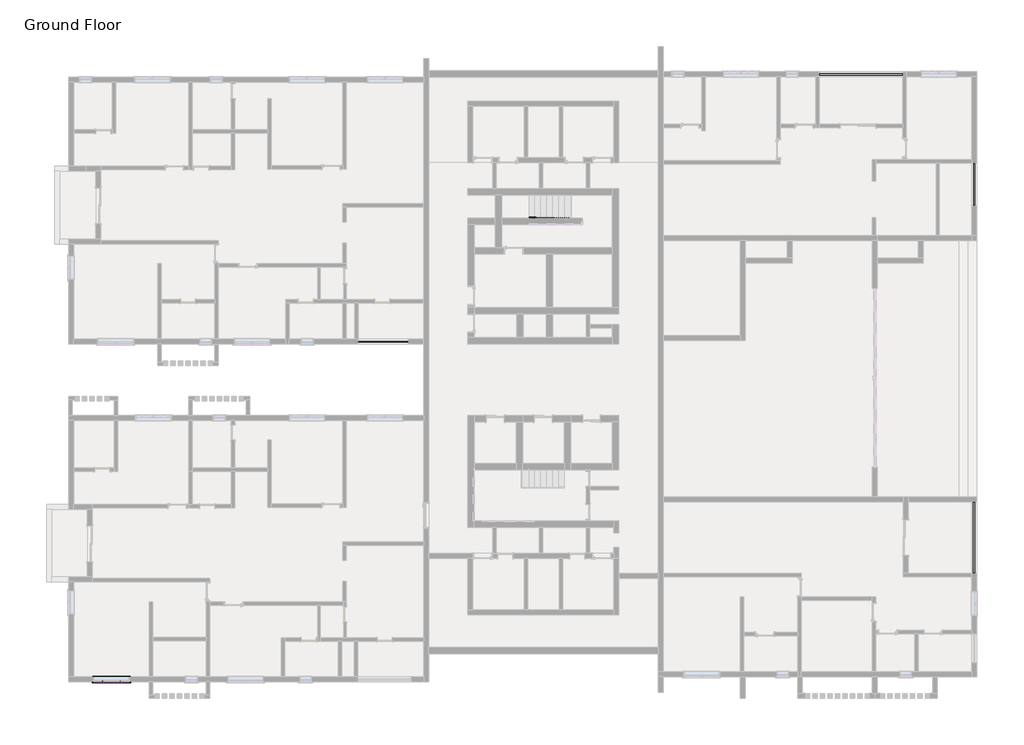
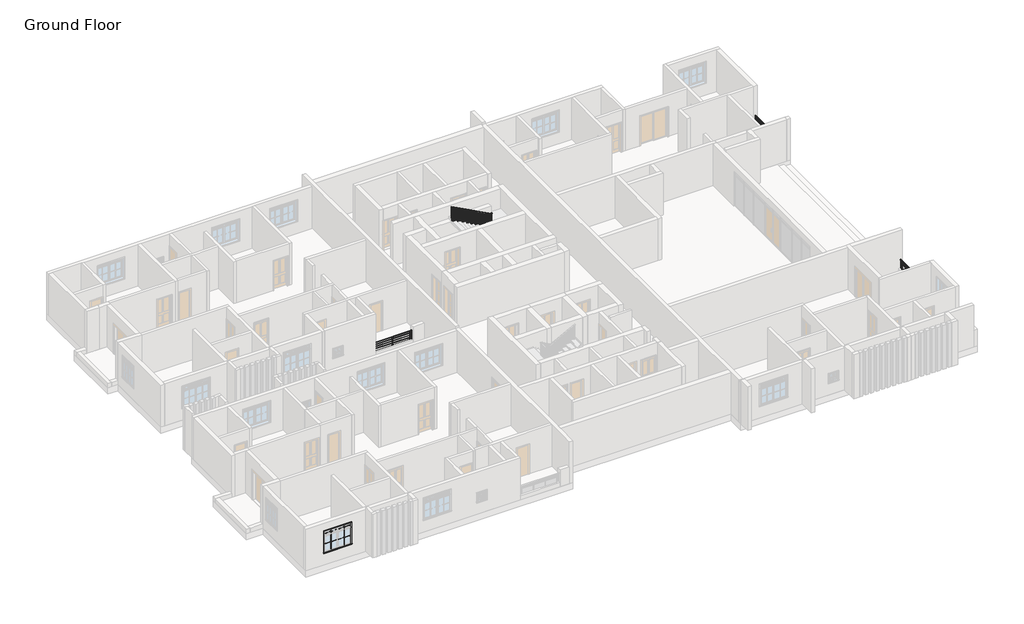
# One storey, part 7 of 9: 6 proxies, 5 railings.
"""IFC4 building model written with IfcOpenShell, lengths in millimetres."""

from ifc_helpers import new_model, si_unit, point, frame, frame_2d, origin, origin_with_axes, place, context, project, spatial, polyline, circle_curve, ellipse_curve, trimmed, segment, composite_curve, outline, extrude, faceted_brep, transform, mapped, element, save
from ifc_brep_helpers import plane_surface, extruded_surface, advanced_brep
from components import muntin_pattern_2x2_muntin_pattern_2x2_dc2504c2, muntin_pattern_2x2_muntin_pattern_2x2_0aa094e9, muntin_pattern_2x2_muntin_pattern_2x2_f17ebf58, trim_window_exterior_flat_with_sill_c22f0c79, trim_window_interior_flat_picture_frame_d1f4d6ef

model = new_model("IFC4")

# Units and contexts
model_context = context("Model", 3, world=origin())
ifc_project = project(units=[si_unit("LENGTHUNIT", "METRE", prefix="MILLI")], contexts=[model_context])

# Site, building, storey
site = spatial("IfcSite", under=ifc_project)
building = spatial("IfcBuilding", under=site)
storey = spatial("IfcBuildingStorey", under=building, Name="Ground Floor", Elevation=0.0)

# Proxies
placement = place(None, origin())
muntin_pattern_2x2_muntin_pattern_2x2_shape = muntin_pattern_2x2_muntin_pattern_2x2_dc2504c2(model_context)
element("IfcBuildingElementProxy", 1, Name="Muntin Pattern_2x2 : Muntin Pattern_2x2", ObjectType="Muntin Pattern_2x2 : Muntin Pattern_2x2", at=placement, inside=storey, context=model_context, shape_type="MappedRepresentation", body=[
    mapped(muntin_pattern_2x2_muntin_pattern_2x2_shape, transform((-11745.8828682, -1988.440108, 984.25), x_axis=(-1.0, 0.0, 0.0), y_axis=(0.0, -1.0, 0.0), z_axis=(0.0, 0.0, 1.0))),
])
muntin_pattern_2x2_muntin_pattern_2x2_2_shape = muntin_pattern_2x2_muntin_pattern_2x2_0aa094e9(model_context)
element("IfcBuildingElementProxy", 2, Name="Muntin Pattern_2x2 : Muntin Pattern_2x2", ObjectType="Muntin Pattern_2x2 : Muntin Pattern_2x2", at=placement, inside=storey, context=model_context, shape_type="MappedRepresentation", body=[
    mapped(muntin_pattern_2x2_muntin_pattern_2x2_2_shape, transform((-12657.1078682, -1988.440108, 984.25), x_axis=(1.0, 0.0, 0.0), y_axis=(0.0, 1.0, 0.0), z_axis=(0.0, 0.0, 1.0))),
])
muntin_pattern_2x2_muntin_pattern_2x2_3_shape = muntin_pattern_2x2_muntin_pattern_2x2_f17ebf58(model_context)
element("IfcBuildingElementProxy", 3, Name="Muntin Pattern_2x2 : Muntin Pattern_2x2", ObjectType="Muntin Pattern_2x2 : Muntin Pattern_2x2", at=placement, inside=storey, context=model_context, shape_type="MappedRepresentation", body=[
    mapped(muntin_pattern_2x2_muntin_pattern_2x2_3_shape, transform((-12657.1078682, -1988.440108, 2203.45), x_axis=(1.0, 0.0, 0.0), y_axis=(0.0, 1.0, 0.0), z_axis=(0.0, 0.0, 1.0))),
])
element("IfcBuildingElementProxy", 4, Name="Muntin Pattern_2x2 : Muntin Pattern_2x2", ObjectType="Muntin Pattern_2x2 : Muntin Pattern_2x2", at=placement, inside=storey, context=model_context, shape_type="MappedRepresentation", body=[
    mapped(muntin_pattern_2x2_muntin_pattern_2x2_3_shape, transform((-11745.8828682, -1988.440108, 2203.45), x_axis=(1.0, 0.0, 0.0), y_axis=(0.0, 1.0, 0.0), z_axis=(0.0, 0.0, 1.0))),
])
trim_window_exterior_flat_with_sill_shape = trim_window_exterior_flat_with_sill_c22f0c79(model_context)
element("IfcBuildingElementProxy", 5, Name="Trim-Window-Exterior-Flat : with Sill", ObjectType="Trim-Window-Exterior-Flat : with Sill", at=placement, inside=storey, context=model_context, shape_type="MappedRepresentation", body=[
    mapped(trim_window_exterior_flat_with_sill_shape, transform((-12201.4953682, -1997.965108, 2438.4), x_axis=(1.0, 0.0, 0.0), y_axis=(0.0, 0.0, 1.0), z_axis=(0.0, -1.0, 0.0))),
])
trim_window_interior_flat_picture_frame_shape = trim_window_interior_flat_picture_frame_d1f4d6ef(model_context)
element("IfcBuildingElementProxy", 6, Name="Trim-Window-Interior-Flat : Picture Frame", ObjectType="Trim-Window-Interior-Flat : Picture Frame", at=placement, inside=storey, context=model_context, shape_type="MappedRepresentation", body=[
    mapped(trim_window_interior_flat_picture_frame_shape, transform((-12201.4953682, -1743.965108, 2438.4), x_axis=(-1.0, 0.0, 0.0), y_axis=(0.0, 0.0, 1.0), z_axis=(0.0, 1.0, 0.0))),
])

# Railings
element("IfcRailing", 7, ObjectType="Glass Panel - Bottom Fill", at=placement, inside=storey, context=model_context, shape_type="SolidModel", body=[
    advanced_brep(
    [(31988.1546318, 7222.234892, 914.4), (31911.9546318, 7222.234892, 914.4), (31988.1546318, 3564.634892, 914.4), (31911.9546318, 3564.634892, 914.4)],
    [
        (0, 1, ellipse_curve(frame((31950.0546318, 7222.234892, 914.4), z_axis=(0.0, 1.0, 0.0), x_axis=(-1.0, 0.0, 0.0)), 38.1, 28.575)),
        (1, 0, ellipse_curve(frame((31950.0546318, 7222.234892, 914.4), z_axis=(0.0, 1.0, 0.0), x_axis=(-1.0, 0.0, 0.0)), 38.1, 28.575)),
        (2, 3, ellipse_curve(frame((31950.0546318, 3564.634892, 914.4), z_axis=(0.0, -1.0, 0.0), x_axis=(-1.0, 0.0, 0.0)), 38.1, 28.575)),
        (3, 2, ellipse_curve(frame((31950.0546318, 3564.634892, 914.4), z_axis=(0.0, -1.0, 0.0), x_axis=(-1.0, 0.0, 0.0)), 38.1, 28.575)),
        (0, 2),
        (3, 1),
    ],
    [
        plane_surface(frame((31950.0546318, 7222.234892, 914.4), z_axis=(0.0, 1.0, 0.0), x_axis=(0.0, 0.0, -1.0))),
        plane_surface(frame((31950.0546318, 3564.634892, 914.4), z_axis=(0.0, -1.0, 0.0), x_axis=(0.0, 0.0, -1.0))),
        extruded_surface(trimmed(ellipse_curve(frame((31950.0546318, 3564.634892, 914.4), z_axis=(0.0, 1.0, 0.0), x_axis=(-1.0, 0.0, 0.0)), 38.1, 28.575), [point((31988.1546318, 3564.634892, 914.4))], [point((31911.9546318, 3564.634892, 914.4))], True, "CARTESIAN"), (0.0, 3657.6000000000004, 0.0), 3657.6000000000004),
        extruded_surface(trimmed(ellipse_curve(frame((31950.0546318, 3564.634892, 914.4), z_axis=(0.0, 1.0, 0.0), x_axis=(-1.0, 0.0, 0.0)), 38.1, 28.575), [point((31911.9546318, 3564.634892, 914.4))], [point((31988.1546318, 3564.634892, 914.4))], True, "CARTESIAN"), (0.0, 3657.6000000000004, 0.0), 3657.6000000000004),
    ],
    [
        (0, [[1, 2]]),
        (1, [[3, 4]]),
        (2, [[-1, 5, -4, 6]]),
        (3, [[-2, -6, -3, -5]]),
    ],
),
    extrude(outline(polyline([(31937.3546318, 7222.234892), (31962.7546318, 7222.234892), (31962.7546318, 3564.634892), (31937.3546318, 3564.634892), (31937.3546318, 7222.234892)])), frame((0.0, 0.0, 800.1), z_axis=(0.0, 0.0, 1.0), x_axis=(1.0, 0.0, 0.0)), (0.0, 0.0, 1.0), 25.4),
    extrude(outline(polyline([(31937.3546318, 7222.234892), (31962.7546318, 7222.234892), (31962.7546318, 3564.634892), (31937.3546318, 3564.634892), (31937.3546318, 7222.234892)])), frame((0.0, 0.0, 698.5), z_axis=(0.0, 0.0, 1.0), x_axis=(1.0, 0.0, 0.0)), (0.0, 0.0, 1.0), 25.4),
    extrude(outline(polyline([(31924.6546318, 3774.184892), (31975.4546318, 3774.184892), (31975.4546318, 3761.484892), (31924.6546318, 3761.484892), (31924.6546318, 3774.184892)])), origin_with_axes(), (0.0, 0.0, 1.0), 885.825),
    extrude(outline(polyline([(31956.5897888, 4580.634892), (31956.5897888, 3767.834892), (31950.2397888, 3767.834892), (31950.2397888, 4580.634892), (31956.5897888, 4580.634892)])), frame((0.0, 0.0, 101.6), z_axis=(0.0, 0.0, 1.0), x_axis=(1.0, 0.0, 0.0)), (0.0, 0.0, 1.0), 596.9),
    extrude(outline(polyline([(31924.6546318, 4586.984892), (31975.4546318, 4586.984892), (31975.4546318, 4574.284892), (31924.6546318, 4574.284892), (31924.6546318, 4586.984892)])), origin_with_axes(), (0.0, 0.0, 1.0), 885.825),
    extrude(outline(polyline([(31956.5897888, 5393.434892), (31956.5897888, 4580.634892), (31950.2397888, 4580.634892), (31950.2397888, 5393.434892), (31956.5897888, 5393.434892)])), frame((0.0, 0.0, 101.6), z_axis=(0.0, 0.0, 1.0), x_axis=(1.0, 0.0, 0.0)), (0.0, 0.0, 1.0), 596.9),
    extrude(outline(polyline([(31924.6546318, 5399.784892), (31975.4546318, 5399.784892), (31975.4546318, 5387.084892), (31924.6546318, 5387.084892), (31924.6546318, 5399.784892)])), origin_with_axes(), (0.0, 0.0, 1.0), 885.825),
    extrude(outline(polyline([(31956.5897888, 6206.234892), (31956.5897888, 5393.434892), (31950.2397888, 5393.434892), (31950.2397888, 6206.234892), (31956.5897888, 6206.234892)])), frame((0.0, 0.0, 101.6), z_axis=(0.0, 0.0, 1.0), x_axis=(1.0, 0.0, 0.0)), (0.0, 0.0, 1.0), 596.9),
    extrude(outline(polyline([(31924.6546318, 6212.584892), (31975.4546318, 6212.584892), (31975.4546318, 6199.884892), (31924.6546318, 6199.884892), (31924.6546318, 6212.584892)])), origin_with_axes(), (0.0, 0.0, 1.0), 885.825),
    extrude(outline(polyline([(31956.5897888, 7019.034892), (31956.5897888, 6206.234892), (31950.2397888, 6206.234892), (31950.2397888, 7019.034892), (31956.5897888, 7019.034892)])), frame((0.0, 0.0, 101.6), z_axis=(0.0, 0.0, 1.0), x_axis=(1.0, 0.0, 0.0)), (0.0, 0.0, 1.0), 596.9),
    extrude(outline(polyline([(31924.6546318, 7025.384892), (31975.4546318, 7025.384892), (31975.4546318, 7012.684892), (31924.6546318, 7012.684892), (31924.6546318, 7025.384892)])), origin_with_axes(), (0.0, 0.0, 1.0), 885.825),
    extrude(outline(polyline([(31940.5296318, 3577.334892), (31959.5796318, 3577.334892), (31959.5796318, 3558.284892), (31940.5296318, 3558.284892), (31940.5296318, 3577.334892)])), origin_with_axes(), (0.0, 0.0, 1.0), 885.825),
    extrude(outline(polyline([(31940.5296318, 7228.584892), (31959.5796318, 7228.584892), (31959.5796318, 7209.534892), (31940.5296318, 7209.534892), (31940.5296318, 7228.584892)])), origin_with_axes(), (0.0, 0.0, 1.0), 885.825),
])
element("IfcRailing", 8, ObjectType="Glass Panel - Bottom Fill", at=placement, inside=storey, context=model_context, shape_type="SolidModel", body=[
    advanced_brep(
    [(23936.3546318, 29155.134892, 914.4), (23936.3546318, 29078.934892, 914.4), (28292.4546318, 29155.134892, 914.4), (28292.4546318, 29078.934892, 914.4)],
    [
        (0, 1, ellipse_curve(frame((23936.3546318, 29117.034892, 914.4), z_axis=(-1.0, 0.0, 0.0), x_axis=(0.0, -1.0, 0.0)), 38.1, 28.575)),
        (1, 0, ellipse_curve(frame((23936.3546318, 29117.034892, 914.4), z_axis=(-1.0, 0.0, 0.0), x_axis=(0.0, -1.0, 0.0)), 38.1, 28.575)),
        (2, 3, ellipse_curve(frame((28292.4546318, 29117.034892, 914.4), z_axis=(1.0, 0.0, 0.0), x_axis=(0.0, -1.0, 0.0)), 38.1, 28.575)),
        (3, 2, ellipse_curve(frame((28292.4546318, 29117.034892, 914.4), z_axis=(1.0, 0.0, 0.0), x_axis=(0.0, -1.0, 0.0)), 38.1, 28.575)),
        (0, 2),
        (3, 1),
    ],
    [
        plane_surface(frame((23936.3546318, 29117.034892, 914.4), z_axis=(-1.0, 0.0, 0.0), x_axis=(0.0, 1.0, 0.0))),
        plane_surface(frame((28292.4546318, 29117.034892, 914.4), z_axis=(1.0, 0.0, 0.0), x_axis=(0.0, 1.0, 0.0))),
        extruded_surface(trimmed(ellipse_curve(frame((28292.4546318, 29117.034892, 914.4), z_axis=(-1.0, 0.0, 0.0), x_axis=(0.0, -1.0, 0.0)), 38.1, 28.575), [point((28292.4546318, 29155.134892, 914.4))], [point((28292.4546318, 29078.934892, 914.4))], True, "CARTESIAN"), (-4356.0999999999985, 0.0, 0.0), 4356.0999999999985),
        extruded_surface(trimmed(ellipse_curve(frame((28292.4546318, 29117.034892, 914.4), z_axis=(-1.0, 0.0, 0.0), x_axis=(0.0, -1.0, 0.0)), 38.1, 28.575), [point((28292.4546318, 29078.934892, 914.4))], [point((28292.4546318, 29155.134892, 914.4))], True, "CARTESIAN"), (-4356.0999999999985, 0.0, 0.0), 4356.0999999999985),
    ],
    [
        (0, [[1, 2]]),
        (1, [[3, 4]]),
        (2, [[-1, 5, -4, 6]]),
        (3, [[-2, -6, -3, -5]]),
    ],
),
    extrude(outline(polyline([(23936.3546318, 29104.334892), (23936.3546318, 29129.734892), (28292.4546318, 29129.734892), (28292.4546318, 29104.334892), (23936.3546318, 29104.334892)])), frame((0.0, 0.0, 800.1), z_axis=(0.0, 0.0, 1.0), x_axis=(1.0, 0.0, 0.0)), (0.0, 0.0, 1.0), 25.4),
    extrude(outline(polyline([(23936.3546318, 29104.334892), (23936.3546318, 29129.734892), (28292.4546318, 29129.734892), (28292.4546318, 29104.334892), (23936.3546318, 29104.334892)])), frame((0.0, 0.0, 698.5), z_axis=(0.0, 0.0, 1.0), x_axis=(1.0, 0.0, 0.0)), (0.0, 0.0, 1.0), 25.4),
    extrude(outline(polyline([(28140.0546318, 29091.634892), (28140.0546318, 29142.434892), (28152.7546318, 29142.434892), (28152.7546318, 29091.634892), (28140.0546318, 29091.634892)])), origin_with_axes(), (0.0, 0.0, 1.0), 885.825),
    extrude(outline(polyline([(27333.6046318, 29123.570049), (28146.4046318, 29123.570049), (28146.4046318, 29117.220049), (27333.6046318, 29117.220049), (27333.6046318, 29123.570049)])), frame((0.0, 0.0, 101.6), z_axis=(0.0, 0.0, 1.0), x_axis=(1.0, 0.0, 0.0)), (0.0, 0.0, 1.0), 596.9),
    extrude(outline(polyline([(27327.2546318, 29091.634892), (27327.2546318, 29142.434892), (27339.9546318, 29142.434892), (27339.9546318, 29091.634892), (27327.2546318, 29091.634892)])), origin_with_axes(), (0.0, 0.0, 1.0), 885.825),
    extrude(outline(polyline([(26520.8046318, 29123.570049), (27333.6046318, 29123.570049), (27333.6046318, 29117.220049), (26520.8046318, 29117.220049), (26520.8046318, 29123.570049)])), frame((0.0, 0.0, 101.6), z_axis=(0.0, 0.0, 1.0), x_axis=(1.0, 0.0, 0.0)), (0.0, 0.0, 1.0), 596.9),
    extrude(outline(polyline([(26514.4546318, 29091.634892), (26514.4546318, 29142.434892), (26527.1546318, 29142.434892), (26527.1546318, 29091.634892), (26514.4546318, 29091.634892)])), origin_with_axes(), (0.0, 0.0, 1.0), 885.825),
    extrude(outline(polyline([(25708.0046318, 29123.570049), (26520.8046318, 29123.570049), (26520.8046318, 29117.220049), (25708.0046318, 29117.220049), (25708.0046318, 29123.570049)])), frame((0.0, 0.0, 101.6), z_axis=(0.0, 0.0, 1.0), x_axis=(1.0, 0.0, 0.0)), (0.0, 0.0, 1.0), 596.9),
    extrude(outline(polyline([(25701.6546318, 29091.634892), (25701.6546318, 29142.434892), (25714.3546318, 29142.434892), (25714.3546318, 29091.634892), (25701.6546318, 29091.634892)])), origin_with_axes(), (0.0, 0.0, 1.0), 885.825),
    extrude(outline(polyline([(24895.2046318, 29123.570049), (25708.0046318, 29123.570049), (25708.0046318, 29117.220049), (24895.2046318, 29117.220049), (24895.2046318, 29123.570049)])), frame((0.0, 0.0, 101.6), z_axis=(0.0, 0.0, 1.0), x_axis=(1.0, 0.0, 0.0)), (0.0, 0.0, 1.0), 596.9),
    extrude(outline(polyline([(24888.8546318, 29091.634892), (24888.8546318, 29142.434892), (24901.5546318, 29142.434892), (24901.5546318, 29091.634892), (24888.8546318, 29091.634892)])), origin_with_axes(), (0.0, 0.0, 1.0), 885.825),
    extrude(outline(polyline([(24082.4046318, 29123.570049), (24895.2046318, 29123.570049), (24895.2046318, 29117.220049), (24082.4046318, 29117.220049), (24082.4046318, 29123.570049)])), frame((0.0, 0.0, 101.6), z_axis=(0.0, 0.0, 1.0), x_axis=(1.0, 0.0, 0.0)), (0.0, 0.0, 1.0), 596.9),
    extrude(outline(polyline([(24076.0546318, 29091.634892), (24076.0546318, 29142.434892), (24088.7546318, 29142.434892), (24088.7546318, 29091.634892), (24076.0546318, 29091.634892)])), origin_with_axes(), (0.0, 0.0, 1.0), 885.825),
    extrude(outline(polyline([(28279.7546318, 29107.509892), (28279.7546318, 29126.559892), (28298.8046318, 29126.559892), (28298.8046318, 29107.509892), (28279.7546318, 29107.509892)])), origin_with_axes(), (0.0, 0.0, 1.0), 885.825),
    extrude(outline(polyline([(23930.0046318, 29107.509892), (23930.0046318, 29126.559892), (23949.0546318, 29126.559892), (23949.0546318, 29107.509892), (23930.0046318, 29107.509892)])), origin_with_axes(), (0.0, 0.0, 1.0), 885.825),
])
element("IfcRailing", 9, ObjectType="Handrail - Pipe", at=placement, inside=storey, context=model_context, shape_type="SweptSolid", body=[
    extrude(outline(composite_curve([segment(trimmed(circle_curve(frame_2d((15426.434892, 895.35)), 19.05), [point((15407.384892, 895.35))], [point((15445.484892, 895.35))], False, "CARTESIAN"), True, "CONTINUOUS"), segment(trimmed(circle_curve(frame_2d((15426.434892, 895.35)), 19.05), [point((15445.484892, 895.35))], [point((15407.384892, 895.35))], False, "CARTESIAN"), True, "CONTINUOUS")], self_intersect=False)), frame((428.6546318, 0.0, 0.0), z_axis=(1.0, 0.0, 0.0), x_axis=(0.0, 1.0, 0.0)), (0.0, 0.0, 1.0), 2565.4),
    extrude(outline(composite_curve([segment(trimmed(circle_curve(frame_2d((15426.434892, 749.3)), 12.7), [point((15439.134892, 749.3))], [point((15413.734892, 749.3))], False, "CARTESIAN"), True, "CONTINUOUS"), segment(trimmed(circle_curve(frame_2d((15426.434892, 749.3)), 12.7), [point((15413.734892, 749.3))], [point((15439.134892, 749.3))], False, "CARTESIAN"), True, "CONTINUOUS")], self_intersect=False)), frame((428.6546318, 0.0, 0.0), z_axis=(1.0, 0.0, 0.0), x_axis=(0.0, 1.0, 0.0)), (0.0, 0.0, 1.0), 2565.4),
    extrude(outline(composite_curve([segment(trimmed(circle_curve(frame_2d((15426.434892, 596.9)), 12.7), [point((15439.134892, 596.9))], [point((15413.734892, 596.9))], False, "CARTESIAN"), True, "CONTINUOUS"), segment(trimmed(circle_curve(frame_2d((15426.434892, 596.9)), 12.7), [point((15413.734892, 596.9))], [point((15439.134892, 596.9))], False, "CARTESIAN"), True, "CONTINUOUS")], self_intersect=False)), frame((428.6546318, 0.0, 0.0), z_axis=(1.0, 0.0, 0.0), x_axis=(0.0, 1.0, 0.0)), (0.0, 0.0, 1.0), 2565.4),
    extrude(outline(composite_curve([segment(trimmed(circle_curve(frame_2d((15426.434892, 444.5)), 12.7), [point((15439.134892, 444.5))], [point((15413.734892, 444.5))], False, "CARTESIAN"), True, "CONTINUOUS"), segment(trimmed(circle_curve(frame_2d((15426.434892, 444.5)), 12.7), [point((15413.734892, 444.5))], [point((15439.134892, 444.5))], False, "CARTESIAN"), True, "CONTINUOUS")], self_intersect=False)), frame((428.6546318, 0.0, 0.0), z_axis=(1.0, 0.0, 0.0), x_axis=(0.0, 1.0, 0.0)), (0.0, 0.0, 1.0), 2565.4),
    extrude(outline(composite_curve([segment(trimmed(circle_curve(frame_2d((15426.434892, 292.1)), 12.7), [point((15439.134892, 292.1))], [point((15413.734892, 292.1))], False, "CARTESIAN"), True, "CONTINUOUS"), segment(trimmed(circle_curve(frame_2d((15426.434892, 292.1)), 12.7), [point((15413.734892, 292.1))], [point((15439.134892, 292.1))], False, "CARTESIAN"), True, "CONTINUOUS")], self_intersect=False)), frame((428.6546318, 0.0, 0.0), z_axis=(1.0, 0.0, 0.0), x_axis=(0.0, 1.0, 0.0)), (0.0, 0.0, 1.0), 2565.4),
    extrude(outline(composite_curve([segment(trimmed(circle_curve(frame_2d((15426.434892, 139.7)), 12.7), [point((15439.134892, 139.7))], [point((15413.734892, 139.7))], False, "CARTESIAN"), True, "CONTINUOUS"), segment(trimmed(circle_curve(frame_2d((15426.434892, 139.7)), 12.7), [point((15413.734892, 139.7))], [point((15439.134892, 139.7))], False, "CARTESIAN"), True, "CONTINUOUS")], self_intersect=False)), frame((428.6546318, 0.0, 0.0), z_axis=(1.0, 0.0, 0.0), x_axis=(0.0, 1.0, 0.0)), (0.0, 0.0, 1.0), 2565.4),
    extrude(outline(composite_curve([segment(trimmed(circle_curve(frame_2d((2867.0546318, 15426.434892)), 12.7), [point((2867.0546318, 15439.134892))], [point((2867.0546318, 15413.734892))], False, "CARTESIAN"), True, "CONTINUOUS"), segment(trimmed(circle_curve(frame_2d((2867.0546318, 15426.434892)), 12.7), [point((2867.0546318, 15413.734892))], [point((2867.0546318, 15439.134892))], False, "CARTESIAN"), True, "CONTINUOUS")], self_intersect=False)), origin_with_axes(), (0.0, 0.0, 1.0), 876.3),
    extrude(outline(composite_curve([segment(trimmed(circle_curve(frame_2d((1647.8546318, 15426.434892)), 12.7), [point((1647.8546318, 15439.134892))], [point((1647.8546318, 15413.734892))], False, "CARTESIAN"), True, "CONTINUOUS"), segment(trimmed(circle_curve(frame_2d((1647.8546318, 15426.434892)), 12.7), [point((1647.8546318, 15413.734892))], [point((1647.8546318, 15439.134892))], False, "CARTESIAN"), True, "CONTINUOUS")], self_intersect=False)), origin_with_axes(), (0.0, 0.0, 1.0), 876.3),
    extrude(outline(composite_curve([segment(trimmed(circle_curve(frame_2d((2981.3546318, 15426.434892)), 12.7), [point((2981.3546318, 15439.134892))], [point((2981.3546318, 15413.734892))], False, "CARTESIAN"), True, "CONTINUOUS"), segment(trimmed(circle_curve(frame_2d((2981.3546318, 15426.434892)), 12.7), [point((2981.3546318, 15413.734892))], [point((2981.3546318, 15439.134892))], False, "CARTESIAN"), True, "CONTINUOUS")], self_intersect=False)), origin_with_axes(), (0.0, 0.0, 1.0), 876.3),
    extrude(outline(composite_curve([segment(trimmed(circle_curve(frame_2d((441.3546318, 15426.434892)), 12.7), [point((441.3546318, 15439.134892))], [point((441.3546318, 15413.734892))], False, "CARTESIAN"), True, "CONTINUOUS"), segment(trimmed(circle_curve(frame_2d((441.3546318, 15426.434892)), 12.7), [point((441.3546318, 15413.734892))], [point((441.3546318, 15439.134892))], False, "CARTESIAN"), True, "CONTINUOUS")], self_intersect=False)), origin_with_axes(), (0.0, 0.0, 1.0), 876.3),
])
element("IfcRailing", 10, ObjectType="Handrail - Pipe", at=placement, inside=storey, context=model_context, shape_type="SweptSolid", body=[
    extrude(outline(composite_curve([segment(trimmed(circle_curve(frame_2d((895.35, 31950.0546318)), 19.05), [point((895.35, 31931.0046318))], [point((895.35, 31969.1046318))], False, "CARTESIAN"), True, "CONTINUOUS"), segment(trimmed(circle_curve(frame_2d((895.35, 31950.0546318)), 19.05), [point((895.35, 31969.1046318))], [point((895.35, 31931.0046318))], False, "CARTESIAN"), True, "CONTINUOUS")], self_intersect=False)), frame((0.0, 22386.034892, 0.0), z_axis=(0.0, 1.0, 0.0), x_axis=(0.0, 0.0, 1.0)), (0.0, 0.0, 1.0), 2184.4),
    extrude(outline(composite_curve([segment(trimmed(circle_curve(frame_2d((749.3, 31950.0546318)), 12.7), [point((749.3, 31962.7546318))], [point((749.3, 31937.3546318))], False, "CARTESIAN"), True, "CONTINUOUS"), segment(trimmed(circle_curve(frame_2d((749.3, 31950.0546318)), 12.7), [point((749.3, 31937.3546318))], [point((749.3, 31962.7546318))], False, "CARTESIAN"), True, "CONTINUOUS")], self_intersect=False)), frame((0.0, 22386.034892, 0.0), z_axis=(0.0, 1.0, 0.0), x_axis=(0.0, 0.0, 1.0)), (0.0, 0.0, 1.0), 2184.4),
    extrude(outline(composite_curve([segment(trimmed(circle_curve(frame_2d((596.9, 31950.0546318)), 12.7), [point((596.9, 31962.7546318))], [point((596.9, 31937.3546318))], False, "CARTESIAN"), True, "CONTINUOUS"), segment(trimmed(circle_curve(frame_2d((596.9, 31950.0546318)), 12.7), [point((596.9, 31937.3546318))], [point((596.9, 31962.7546318))], False, "CARTESIAN"), True, "CONTINUOUS")], self_intersect=False)), frame((0.0, 22386.034892, 0.0), z_axis=(0.0, 1.0, 0.0), x_axis=(0.0, 0.0, 1.0)), (0.0, 0.0, 1.0), 2184.4),
    extrude(outline(composite_curve([segment(trimmed(circle_curve(frame_2d((444.5, 31950.0546318)), 12.7), [point((444.5, 31962.7546318))], [point((444.5, 31937.3546318))], False, "CARTESIAN"), True, "CONTINUOUS"), segment(trimmed(circle_curve(frame_2d((444.5, 31950.0546318)), 12.7), [point((444.5, 31937.3546318))], [point((444.5, 31962.7546318))], False, "CARTESIAN"), True, "CONTINUOUS")], self_intersect=False)), frame((0.0, 22386.034892, 0.0), z_axis=(0.0, 1.0, 0.0), x_axis=(0.0, 0.0, 1.0)), (0.0, 0.0, 1.0), 2184.4),
    extrude(outline(composite_curve([segment(trimmed(circle_curve(frame_2d((292.1, 31950.0546318)), 12.7), [point((292.1, 31962.7546318))], [point((292.1, 31937.3546318))], False, "CARTESIAN"), True, "CONTINUOUS"), segment(trimmed(circle_curve(frame_2d((292.1, 31950.0546318)), 12.7), [point((292.1, 31937.3546318))], [point((292.1, 31962.7546318))], False, "CARTESIAN"), True, "CONTINUOUS")], self_intersect=False)), frame((0.0, 22386.034892, 0.0), z_axis=(0.0, 1.0, 0.0), x_axis=(0.0, 0.0, 1.0)), (0.0, 0.0, 1.0), 2184.4),
    extrude(outline(composite_curve([segment(trimmed(circle_curve(frame_2d((139.7, 31950.0546318)), 12.7), [point((139.7, 31962.7546318))], [point((139.7, 31937.3546318))], False, "CARTESIAN"), True, "CONTINUOUS"), segment(trimmed(circle_curve(frame_2d((139.7, 31950.0546318)), 12.7), [point((139.7, 31937.3546318))], [point((139.7, 31962.7546318))], False, "CARTESIAN"), True, "CONTINUOUS")], self_intersect=False)), frame((0.0, 22386.034892, 0.0), z_axis=(0.0, 1.0, 0.0), x_axis=(0.0, 0.0, 1.0)), (0.0, 0.0, 1.0), 2184.4),
    extrude(outline(composite_curve([segment(trimmed(circle_curve(frame_2d((31950.0546318, 23351.234892)), 12.7), [point((31962.7546318, 23351.234892))], [point((31937.3546318, 23351.234892))], False, "CARTESIAN"), True, "CONTINUOUS"), segment(trimmed(circle_curve(frame_2d((31950.0546318, 23351.234892)), 12.7), [point((31937.3546318, 23351.234892))], [point((31962.7546318, 23351.234892))], False, "CARTESIAN"), True, "CONTINUOUS")], self_intersect=False)), origin_with_axes(), (0.0, 0.0, 1.0), 876.3),
    extrude(outline(composite_curve([segment(trimmed(circle_curve(frame_2d((31950.0546318, 22398.734892)), 12.7), [point((31962.7546318, 22398.734892))], [point((31937.3546318, 22398.734892))], False, "CARTESIAN"), True, "CONTINUOUS"), segment(trimmed(circle_curve(frame_2d((31950.0546318, 22398.734892)), 12.7), [point((31937.3546318, 22398.734892))], [point((31962.7546318, 22398.734892))], False, "CARTESIAN"), True, "CONTINUOUS")], self_intersect=False)), origin_with_axes(), (0.0, 0.0, 1.0), 876.3),
    extrude(outline(composite_curve([segment(trimmed(circle_curve(frame_2d((31950.0546318, 24557.734892)), 12.7), [point((31962.7546318, 24557.734892))], [point((31937.3546318, 24557.734892))], False, "CARTESIAN"), True, "CONTINUOUS"), segment(trimmed(circle_curve(frame_2d((31950.0546318, 24557.734892)), 12.7), [point((31937.3546318, 24557.734892))], [point((31962.7546318, 24557.734892))], False, "CARTESIAN"), True, "CONTINUOUS")], self_intersect=False)), origin_with_axes(), (0.0, 0.0, 1.0), 876.3),
])
element("IfcRailing", 11, ObjectType="Handrail - Rectangular", at=placement, inside=storey, context=model_context, shape_type="SolidModel", body=[
    faceted_brep([(9166.2546318, 21801.834892, 1074.42), (9166.2546318, 21801.834892, 1017.0446664), (9166.2546318, 21751.034892, 1017.0446664), (9166.2546318, 21751.034892, 1074.42), (11833.2546318, 21801.834892, 2474.595), (11884.0546318, 21801.834892, 2443.8896664), (11884.0546318, 21751.034892, 2443.8896664), (11833.2546318, 21751.034892, 2474.595), (11833.2546318, 21801.834892, 2514.6), (11884.0546318, 21801.834892, 2463.8), (11884.0546318, 21751.034892, 2463.8), (11833.2546318, 21751.034892, 2514.6), (11960.2546318, 21801.834892, 2514.6), (11960.2546318, 21801.834892, 2463.8), (11909.4546318, 21751.034892, 2463.8), (11909.4546318, 21751.034892, 2514.6), (11960.2546318, 21674.834892, 2514.6), (11960.2546318, 21674.834892, 2463.8), (11909.4546318, 21674.834892, 2463.8), (11909.4546318, 21674.834892, 2514.6), (11960.2546318, 21497.034892, 2514.6), (11960.2546318, 21446.234892, 2463.8), (11909.4546318, 21446.234892, 2463.8), (11909.4546318, 21497.034892, 2514.6), (11960.2546318, 21497.034892, 2714.625), (11960.2546318, 21446.234892, 2663.825), (11909.4546318, 21446.234892, 2663.825), (11909.4546318, 21497.034892, 2714.625), (11960.2546318, 21370.034892, 2714.625), (11960.2546318, 21370.034892, 2663.825), (11909.4546318, 21420.834892, 2663.825), (11909.4546318, 21420.834892, 2714.625), (11833.2546318, 21370.034892, 2714.625), (11820.7301869, 21370.034892, 2663.825), (11820.7301869, 21420.834892, 2663.825), (11833.2546318, 21420.834892, 2714.625), (9166.2546318, 21370.034892, 4114.8), (9166.2546318, 21420.834892, 4114.8), (9166.2546318, 21420.834892, 4057.4246664), (9166.2546318, 21370.034892, 4057.4246664)], [[[0, 1, 2, 3]], [[1, 0, 4, 5]], [[2, 1, 5, 6]], [[3, 2, 6, 7]], [[0, 3, 7, 4]], [[5, 4, 8, 9]], [[6, 5, 9, 10]], [[7, 6, 10, 11]], [[4, 7, 11, 8]], [[9, 8, 12, 13]], [[10, 9, 13, 14]], [[11, 10, 14, 15]], [[8, 11, 15, 12]], [[13, 12, 16, 17]], [[14, 13, 17, 18]], [[15, 14, 18, 19]], [[12, 15, 19, 16]], [[17, 16, 20, 21]], [[18, 17, 21, 22]], [[19, 18, 22, 23]], [[16, 19, 23, 20]], [[21, 20, 24, 25]], [[22, 21, 25, 26]], [[23, 22, 26, 27]], [[20, 23, 27, 24]], [[25, 24, 28, 29]], [[26, 25, 29, 30]], [[27, 26, 30, 31]], [[24, 27, 31, 28]], [[29, 28, 32, 33]], [[30, 29, 33, 34]], [[31, 30, 34, 35]], [[28, 31, 35, 32]], [[36, 37, 38, 39]], [[33, 32, 36, 39]], [[34, 33, 39, 38]], [[35, 34, 38, 37]], [[32, 35, 37, 36]]]),
    extrude(outline(polyline([(4039.0890414, 9201.1796318), (4049.0902914, 9182.1296318), (3040.38, 9182.1296318), (3040.38, 9201.1796318), (4039.0890414, 9201.1796318)])), frame((0.0, 21385.909892, 0.0), z_axis=(0.0, 1.0, 0.0), x_axis=(0.0, 0.0, 1.0)), (0.0, 0.0, 1.0), 19.05),
    extrude(outline(polyline([(3985.7490414, 9302.7796318), (3995.7502914, 9283.7296318), (3040.38, 9283.7296318), (3040.38, 9302.7796318), (3985.7490414, 9302.7796318)])), frame((0.0, 21385.909892, 0.0), z_axis=(0.0, 1.0, 0.0), x_axis=(0.0, 0.0, 1.0)), (0.0, 0.0, 1.0), 19.05),
    extrude(outline(polyline([(3932.4090414, 9404.3796318), (3942.4102914, 9385.3296318), (3040.38, 9385.3296318), (3040.38, 9404.3796318), (3932.4090414, 9404.3796318)])), frame((0.0, 21385.909892, 0.0), z_axis=(0.0, 1.0, 0.0), x_axis=(0.0, 0.0, 1.0)), (0.0, 0.0, 1.0), 19.05),
    extrude(outline(polyline([(3879.0690414, 9505.9796318), (3889.0702914, 9486.9296318), (2880.36, 9486.9296318), (2880.36, 9505.9796318), (3879.0690414, 9505.9796318)])), frame((0.0, 21385.909892, 0.0), z_axis=(0.0, 1.0, 0.0), x_axis=(0.0, 0.0, 1.0)), (0.0, 0.0, 1.0), 19.05),
    extrude(outline(polyline([(3825.7290414, 9607.5796318), (3835.7302914, 9588.5296318), (2880.36, 9588.5296318), (2880.36, 9607.5796318), (3825.7290414, 9607.5796318)])), frame((0.0, 21385.909892, 0.0), z_axis=(0.0, 1.0, 0.0), x_axis=(0.0, 0.0, 1.0)), (0.0, 0.0, 1.0), 19.05),
    extrude(outline(polyline([(3772.3890414, 9709.1796318), (3782.3902914, 9690.1296318), (2880.36, 9690.1296318), (2880.36, 9709.1796318), (3772.3890414, 9709.1796318)])), frame((0.0, 21385.909892, 0.0), z_axis=(0.0, 1.0, 0.0), x_axis=(0.0, 0.0, 1.0)), (0.0, 0.0, 1.0), 19.05),
    extrude(outline(polyline([(3719.0490414, 9810.7796318), (3729.0502914, 9791.7296318), (2720.34, 9791.7296318), (2720.34, 9810.7796318), (3719.0490414, 9810.7796318)])), frame((0.0, 21385.909892, 0.0), z_axis=(0.0, 1.0, 0.0), x_axis=(0.0, 0.0, 1.0)), (0.0, 0.0, 1.0), 19.05),
    extrude(outline(polyline([(3665.7090414, 9912.3796318), (3675.7102914, 9893.3296318), (2720.34, 9893.3296318), (2720.34, 9912.3796318), (3665.7090414, 9912.3796318)])), frame((0.0, 21385.909892, 0.0), z_axis=(0.0, 1.0, 0.0), x_axis=(0.0, 0.0, 1.0)), (0.0, 0.0, 1.0), 19.05),
    extrude(outline(polyline([(3612.3690414, 10013.9796318), (3622.3702914, 9994.9296318), (2720.34, 9994.9296318), (2720.34, 10013.9796318), (3612.3690414, 10013.9796318)])), frame((0.0, 21385.909892, 0.0), z_axis=(0.0, 1.0, 0.0), x_axis=(0.0, 0.0, 1.0)), (0.0, 0.0, 1.0), 19.05),
    extrude(outline(polyline([(3559.0290414, 10115.5796318), (3569.0302914, 10096.5296318), (2560.32, 10096.5296318), (2560.32, 10115.5796318), (3559.0290414, 10115.5796318)])), frame((0.0, 21385.909892, 0.0), z_axis=(0.0, 1.0, 0.0), x_axis=(0.0, 0.0, 1.0)), (0.0, 0.0, 1.0), 19.05),
    extrude(outline(polyline([(3505.6890414, 10217.1796318), (3515.6902914, 10198.1296318), (2560.32, 10198.1296318), (2560.32, 10217.1796318), (3505.6890414, 10217.1796318)])), frame((0.0, 21385.909892, 0.0), z_axis=(0.0, 1.0, 0.0), x_axis=(0.0, 0.0, 1.0)), (0.0, 0.0, 1.0), 19.05),
    extrude(outline(polyline([(3452.3490414, 10318.7796318), (3462.3502914, 10299.7296318), (2560.32, 10299.7296318), (2560.32, 10318.7796318), (3452.3490414, 10318.7796318)])), frame((0.0, 21385.909892, 0.0), z_axis=(0.0, 1.0, 0.0), x_axis=(0.0, 0.0, 1.0)), (0.0, 0.0, 1.0), 19.05),
    extrude(outline(polyline([(3399.0090414, 10420.3796318), (3409.0102914, 10401.3296318), (2400.3, 10401.3296318), (2400.3, 10420.3796318), (3399.0090414, 10420.3796318)])), frame((0.0, 21385.909892, 0.0), z_axis=(0.0, 1.0, 0.0), x_axis=(0.0, 0.0, 1.0)), (0.0, 0.0, 1.0), 19.05),
    extrude(outline(polyline([(3345.6690414, 10521.9796318), (3355.6702914, 10502.9296318), (2400.3, 10502.9296318), (2400.3, 10521.9796318), (3345.6690414, 10521.9796318)])), frame((0.0, 21385.909892, 0.0), z_axis=(0.0, 1.0, 0.0), x_axis=(0.0, 0.0, 1.0)), (0.0, 0.0, 1.0), 19.05),
    extrude(outline(polyline([(3292.3290414, 10623.5796318), (3302.3302914, 10604.5296318), (2400.3, 10604.5296318), (2400.3, 10623.5796318), (3292.3290414, 10623.5796318)])), frame((0.0, 21385.909892, 0.0), z_axis=(0.0, 1.0, 0.0), x_axis=(0.0, 0.0, 1.0)), (0.0, 0.0, 1.0), 19.05),
    extrude(outline(polyline([(3238.9890414, 10725.1796318), (3248.9902914, 10706.1296318), (2240.28, 10706.1296318), (2240.28, 10725.1796318), (3238.9890414, 10725.1796318)])), frame((0.0, 21385.909892, 0.0), z_axis=(0.0, 1.0, 0.0), x_axis=(0.0, 0.0, 1.0)), (0.0, 0.0, 1.0), 19.05),
    extrude(outline(polyline([(3185.6490414, 10826.7796318), (3195.6502914, 10807.7296318), (2240.28, 10807.7296318), (2240.28, 10826.7796318), (3185.6490414, 10826.7796318)])), frame((0.0, 21385.909892, 0.0), z_axis=(0.0, 1.0, 0.0), x_axis=(0.0, 0.0, 1.0)), (0.0, 0.0, 1.0), 19.05),
    extrude(outline(polyline([(3132.3090414, 10928.3796318), (3142.3102914, 10909.3296318), (2240.28, 10909.3296318), (2240.28, 10928.3796318), (3132.3090414, 10928.3796318)])), frame((0.0, 21385.909892, 0.0), z_axis=(0.0, 1.0, 0.0), x_axis=(0.0, 0.0, 1.0)), (0.0, 0.0, 1.0), 19.05),
    extrude(outline(polyline([(3078.9690414, 11029.9796318), (3088.9702914, 11010.9296318), (2080.26, 11010.9296318), (2080.26, 11029.9796318), (3078.9690414, 11029.9796318)])), frame((0.0, 21385.909892, 0.0), z_axis=(0.0, 1.0, 0.0), x_axis=(0.0, 0.0, 1.0)), (0.0, 0.0, 1.0), 19.05),
    extrude(outline(polyline([(3025.6290414, 11131.5796318), (3035.6302914, 11112.5296318), (2080.26, 11112.5296318), (2080.26, 11131.5796318), (3025.6290414, 11131.5796318)])), frame((0.0, 21385.909892, 0.0), z_axis=(0.0, 1.0, 0.0), x_axis=(0.0, 0.0, 1.0)), (0.0, 0.0, 1.0), 19.05),
    extrude(outline(polyline([(2972.2890414, 11233.1796318), (2982.2902914, 11214.1296318), (2080.26, 11214.1296318), (2080.26, 11233.1796318), (2972.2890414, 11233.1796318)])), frame((0.0, 21385.909892, 0.0), z_axis=(0.0, 1.0, 0.0), x_axis=(0.0, 0.0, 1.0)), (0.0, 0.0, 1.0), 19.05),
    extrude(outline(polyline([(2918.9490414, 11334.7796318), (2928.9502914, 11315.7296318), (1920.24, 11315.7296318), (1920.24, 11334.7796318), (2918.9490414, 11334.7796318)])), frame((0.0, 21385.909892, 0.0), z_axis=(0.0, 1.0, 0.0), x_axis=(0.0, 0.0, 1.0)), (0.0, 0.0, 1.0), 19.05),
    extrude(outline(polyline([(2865.6090414, 11436.3796318), (2875.6102914, 11417.3296318), (1920.24, 11417.3296318), (1920.24, 11436.3796318), (2865.6090414, 11436.3796318)])), frame((0.0, 21385.909892, 0.0), z_axis=(0.0, 1.0, 0.0), x_axis=(0.0, 0.0, 1.0)), (0.0, 0.0, 1.0), 19.05),
    extrude(outline(polyline([(2812.2690414, 11537.9796318), (2822.2702914, 11518.9296318), (1920.24, 11518.9296318), (1920.24, 11537.9796318), (2812.2690414, 11537.9796318)])), frame((0.0, 21385.909892, 0.0), z_axis=(0.0, 1.0, 0.0), x_axis=(0.0, 0.0, 1.0)), (0.0, 0.0, 1.0), 19.05),
    extrude(outline(polyline([(2758.9290414, 11639.5796318), (2768.9302914, 11620.5296318), (1760.22, 11620.5296318), (1760.22, 11639.5796318), (2758.9290414, 11639.5796318)])), frame((0.0, 21385.909892, 0.0), z_axis=(0.0, 1.0, 0.0), x_axis=(0.0, 0.0, 1.0)), (0.0, 0.0, 1.0), 19.05),
    extrude(outline(polyline([(2705.5890414, 11741.1796318), (2715.5902914, 11722.1296318), (1760.22, 11722.1296318), (1760.22, 11741.1796318), (2705.5890414, 11741.1796318)])), frame((0.0, 21385.909892, 0.0), z_axis=(0.0, 1.0, 0.0), x_axis=(0.0, 0.0, 1.0)), (0.0, 0.0, 1.0), 19.05),
    extrude(outline(polyline([(2652.2490414, 11842.7796318), (2662.2502914, 11823.7296318), (1760.22, 11823.7296318), (1760.22, 11842.7796318), (2652.2490414, 11842.7796318)])), frame((0.0, 21385.909892, 0.0), z_axis=(0.0, 1.0, 0.0), x_axis=(0.0, 0.0, 1.0)), (0.0, 0.0, 1.0), 19.05),
    extrude(outline(polyline([(11925.3296318, 21481.159892), (11944.3796318, 21481.159892), (11944.3796318, 21462.109892), (11925.3296318, 21462.109892), (11925.3296318, 21481.159892)])), frame((0.0, 0.0, 1600.2), z_axis=(0.0, 0.0, 1.0), x_axis=(1.0, 0.0, 0.0)), (0.0, 0.0, 1.0), 1063.625),
    extrude(outline(polyline([(11925.3296318, 21582.759892), (11944.3796318, 21582.759892), (11944.3796318, 21563.709892), (11925.3296318, 21563.709892), (11925.3296318, 21582.759892)])), frame((0.0, 0.0, 1600.2), z_axis=(0.0, 0.0, 1.0), x_axis=(1.0, 0.0, 0.0)), (0.0, 0.0, 1.0), 863.6),
    extrude(outline(polyline([(11925.3296318, 21684.359892), (11944.3796318, 21684.359892), (11944.3796318, 21665.309892), (11925.3296318, 21665.309892), (11925.3296318, 21684.359892)])), frame((0.0, 0.0, 1600.2), z_axis=(0.0, 0.0, 1.0), x_axis=(1.0, 0.0, 0.0)), (0.0, 0.0, 1.0), 863.6),
    extrude(outline(polyline([(11899.9296318, 21766.909892), (11899.9296318, 21785.959892), (11918.9796318, 21785.959892), (11918.9796318, 21766.909892), (11899.9296318, 21766.909892)])), frame((0.0, 0.0, 1600.2), z_axis=(0.0, 0.0, 1.0), x_axis=(1.0, 0.0, 0.0)), (0.0, 0.0, 1.0), 863.6),
    extrude(outline(polyline([(2408.8852914, 11817.3796318), (2398.8840414, 11798.3296318), (1440.18, 11798.3296318), (1440.18, 11817.3796318), (2408.8852914, 11817.3796318)])), frame((0.0, 21766.909892, 0.0), z_axis=(0.0, 1.0, 0.0), x_axis=(0.0, 0.0, 1.0)), (0.0, 0.0, 1.0), 19.05),
    extrude(outline(polyline([(2355.5452914, 11715.7796318), (2345.5440414, 11696.7296318), (1440.18, 11696.7296318), (1440.18, 11715.7796318), (2355.5452914, 11715.7796318)])), frame((0.0, 21766.909892, 0.0), z_axis=(0.0, 1.0, 0.0), x_axis=(0.0, 0.0, 1.0)), (0.0, 0.0, 1.0), 19.05),
    extrude(outline(polyline([(2302.2052914, 11614.1796318), (2292.2040414, 11595.1296318), (1440.18, 11595.1296318), (1440.18, 11614.1796318), (2302.2052914, 11614.1796318)])), frame((0.0, 21766.909892, 0.0), z_axis=(0.0, 1.0, 0.0), x_axis=(0.0, 0.0, 1.0)), (0.0, 0.0, 1.0), 19.05),
    extrude(outline(polyline([(2248.8652914, 11512.5796318), (2238.8640414, 11493.5296318), (1280.16, 11493.5296318), (1280.16, 11512.5796318), (2248.8652914, 11512.5796318)])), frame((0.0, 21766.909892, 0.0), z_axis=(0.0, 1.0, 0.0), x_axis=(0.0, 0.0, 1.0)), (0.0, 0.0, 1.0), 19.05),
    extrude(outline(polyline([(2195.5252914, 11410.9796318), (2185.5240414, 11391.9296318), (1280.16, 11391.9296318), (1280.16, 11410.9796318), (2195.5252914, 11410.9796318)])), frame((0.0, 21766.909892, 0.0), z_axis=(0.0, 1.0, 0.0), x_axis=(0.0, 0.0, 1.0)), (0.0, 0.0, 1.0), 19.05),
    extrude(outline(polyline([(2142.1852914, 11309.3796318), (2132.1840414, 11290.3296318), (1280.16, 11290.3296318), (1280.16, 11309.3796318), (2142.1852914, 11309.3796318)])), frame((0.0, 21766.909892, 0.0), z_axis=(0.0, 1.0, 0.0), x_axis=(0.0, 0.0, 1.0)), (0.0, 0.0, 1.0), 19.05),
    extrude(outline(polyline([(2088.8452914, 11207.7796318), (2078.8440414, 11188.7296318), (1120.14, 11188.7296318), (1120.14, 11207.7796318), (2088.8452914, 11207.7796318)])), frame((0.0, 21766.909892, 0.0), z_axis=(0.0, 1.0, 0.0), x_axis=(0.0, 0.0, 1.0)), (0.0, 0.0, 1.0), 19.05),
    extrude(outline(polyline([(2035.5052914, 11106.1796318), (2025.5040414, 11087.1296318), (1120.14, 11087.1296318), (1120.14, 11106.1796318), (2035.5052914, 11106.1796318)])), frame((0.0, 21766.909892, 0.0), z_axis=(0.0, 1.0, 0.0), x_axis=(0.0, 0.0, 1.0)), (0.0, 0.0, 1.0), 19.05),
    extrude(outline(polyline([(1982.1652914, 11004.5796318), (1972.1640414, 10985.5296318), (1120.14, 10985.5296318), (1120.14, 11004.5796318), (1982.1652914, 11004.5796318)])), frame((0.0, 21766.909892, 0.0), z_axis=(0.0, 1.0, 0.0), x_axis=(0.0, 0.0, 1.0)), (0.0, 0.0, 1.0), 19.05),
    extrude(outline(polyline([(1928.8252914, 10902.9796318), (1918.8240414, 10883.9296318), (960.12, 10883.9296318), (960.12, 10902.9796318), (1928.8252914, 10902.9796318)])), frame((0.0, 21766.909892, 0.0), z_axis=(0.0, 1.0, 0.0), x_axis=(0.0, 0.0, 1.0)), (0.0, 0.0, 1.0), 19.05),
    extrude(outline(polyline([(1875.4852914, 10801.3796318), (1865.4840414, 10782.3296318), (960.12, 10782.3296318), (960.12, 10801.3796318), (1875.4852914, 10801.3796318)])), frame((0.0, 21766.909892, 0.0), z_axis=(0.0, 1.0, 0.0), x_axis=(0.0, 0.0, 1.0)), (0.0, 0.0, 1.0), 19.05),
    extrude(outline(polyline([(1822.1452914, 10699.7796318), (1812.1440414, 10680.7296318), (960.12, 10680.7296318), (960.12, 10699.7796318), (1822.1452914, 10699.7796318)])), frame((0.0, 21766.909892, 0.0), z_axis=(0.0, 1.0, 0.0), x_axis=(0.0, 0.0, 1.0)), (0.0, 0.0, 1.0), 19.05),
    extrude(outline(polyline([(1768.8052914, 10598.1796318), (1758.8040414, 10579.1296318), (800.1, 10579.1296318), (800.1, 10598.1796318), (1768.8052914, 10598.1796318)])), frame((0.0, 21766.909892, 0.0), z_axis=(0.0, 1.0, 0.0), x_axis=(0.0, 0.0, 1.0)), (0.0, 0.0, 1.0), 19.05),
    extrude(outline(polyline([(1715.4652914, 10496.5796318), (1705.4640414, 10477.5296318), (800.1, 10477.5296318), (800.1, 10496.5796318), (1715.4652914, 10496.5796318)])), frame((0.0, 21766.909892, 0.0), z_axis=(0.0, 1.0, 0.0), x_axis=(0.0, 0.0, 1.0)), (0.0, 0.0, 1.0), 19.05),
    extrude(outline(polyline([(1662.1252914, 10394.9796318), (1652.1240414, 10375.9296318), (800.1, 10375.9296318), (800.1, 10394.9796318), (1662.1252914, 10394.9796318)])), frame((0.0, 21766.909892, 0.0), z_axis=(0.0, 1.0, 0.0), x_axis=(0.0, 0.0, 1.0)), (0.0, 0.0, 1.0), 19.05),
    extrude(outline(polyline([(1608.7852914, 10293.3796318), (1598.7840414, 10274.3296318), (640.08, 10274.3296318), (640.08, 10293.3796318), (1608.7852914, 10293.3796318)])), frame((0.0, 21766.909892, 0.0), z_axis=(0.0, 1.0, 0.0), x_axis=(0.0, 0.0, 1.0)), (0.0, 0.0, 1.0), 19.05),
    extrude(outline(polyline([(1555.4452914, 10191.7796318), (1545.4440414, 10172.7296318), (640.08, 10172.7296318), (640.08, 10191.7796318), (1555.4452914, 10191.7796318)])), frame((0.0, 21766.909892, 0.0), z_axis=(0.0, 1.0, 0.0), x_axis=(0.0, 0.0, 1.0)), (0.0, 0.0, 1.0), 19.05),
    extrude(outline(polyline([(1502.1052914, 10090.1796318), (1492.1040414, 10071.1296318), (640.08, 10071.1296318), (640.08, 10090.1796318), (1502.1052914, 10090.1796318)])), frame((0.0, 21766.909892, 0.0), z_axis=(0.0, 1.0, 0.0), x_axis=(0.0, 0.0, 1.0)), (0.0, 0.0, 1.0), 19.05),
    extrude(outline(polyline([(1448.7652914, 9988.5796318), (1438.7640414, 9969.5296318), (480.06, 9969.5296318), (480.06, 9988.5796318), (1448.7652914, 9988.5796318)])), frame((0.0, 21766.909892, 0.0), z_axis=(0.0, 1.0, 0.0), x_axis=(0.0, 0.0, 1.0)), (0.0, 0.0, 1.0), 19.05),
    extrude(outline(polyline([(1395.4252914, 9886.9796318), (1385.4240414, 9867.9296318), (480.06, 9867.9296318), (480.06, 9886.9796318), (1395.4252914, 9886.9796318)])), frame((0.0, 21766.909892, 0.0), z_axis=(0.0, 1.0, 0.0), x_axis=(0.0, 0.0, 1.0)), (0.0, 0.0, 1.0), 19.05),
    extrude(outline(polyline([(1342.0852914, 9785.3796318), (1332.0840414, 9766.3296318), (480.06, 9766.3296318), (480.06, 9785.3796318), (1342.0852914, 9785.3796318)])), frame((0.0, 21766.909892, 0.0), z_axis=(0.0, 1.0, 0.0), x_axis=(0.0, 0.0, 1.0)), (0.0, 0.0, 1.0), 19.05),
    extrude(outline(polyline([(1288.7452914, 9683.7796318), (1278.7440414, 9664.7296318), (320.04, 9664.7296318), (320.04, 9683.7796318), (1288.7452914, 9683.7796318)])), frame((0.0, 21766.909892, 0.0), z_axis=(0.0, 1.0, 0.0), x_axis=(0.0, 0.0, 1.0)), (0.0, 0.0, 1.0), 19.05),
    extrude(outline(polyline([(1235.4052914, 9582.1796318), (1225.4040414, 9563.1296318), (320.04, 9563.1296318), (320.04, 9582.1796318), (1235.4052914, 9582.1796318)])), frame((0.0, 21766.909892, 0.0), z_axis=(0.0, 1.0, 0.0), x_axis=(0.0, 0.0, 1.0)), (0.0, 0.0, 1.0), 19.05),
    extrude(outline(polyline([(1182.0652914, 9480.5796318), (1172.0640414, 9461.5296318), (320.04, 9461.5296318), (320.04, 9480.5796318), (1182.0652914, 9480.5796318)])), frame((0.0, 21766.909892, 0.0), z_axis=(0.0, 1.0, 0.0), x_axis=(0.0, 0.0, 1.0)), (0.0, 0.0, 1.0), 19.05),
    extrude(outline(polyline([(1128.7252914, 9378.9796318), (1118.7240414, 9359.9296318), (160.02, 9359.9296318), (160.02, 9378.9796318), (1128.7252914, 9378.9796318)])), frame((0.0, 21766.909892, 0.0), z_axis=(0.0, 1.0, 0.0), x_axis=(0.0, 0.0, 1.0)), (0.0, 0.0, 1.0), 19.05),
    extrude(outline(polyline([(1075.3852914, 9277.3796318), (1065.3840414, 9258.3296318), (160.02, 9258.3296318), (160.02, 9277.3796318), (1075.3852914, 9277.3796318)])), frame((0.0, 21766.909892, 0.0), z_axis=(0.0, 1.0, 0.0), x_axis=(0.0, 0.0, 1.0)), (0.0, 0.0, 1.0), 19.05),
    extrude(outline(polyline([(11925.3296318, 21404.959892), (11944.3796318, 21404.959892), (11944.3796318, 21385.909892), (11925.3296318, 21385.909892), (11925.3296318, 21404.959892)])), frame((0.0, 0.0, 1600.2), z_axis=(0.0, 0.0, 1.0), x_axis=(1.0, 0.0, 0.0)), (0.0, 0.0, 1.0), 1063.625),
    extrude(outline(polyline([(11925.3296318, 21766.909892), (11925.3296318, 21785.959892), (11944.3796318, 21785.959892), (11944.3796318, 21766.909892), (11925.3296318, 21766.909892)])), frame((0.0, 0.0, 1600.2), z_axis=(0.0, 0.0, 1.0), x_axis=(1.0, 0.0, 0.0)), (0.0, 0.0, 1.0), 863.6),
    extrude(outline(polyline([(4047.4234164, 9185.3046318), (4057.4246664, 9166.2546318), (3040.38, 9166.2546318), (3040.38, 9185.3046318), (4047.4234164, 9185.3046318)])), frame((0.0, 21385.909892, 0.0), z_axis=(0.0, 1.0, 0.0), x_axis=(0.0, 0.0, 1.0)), (0.0, 0.0, 1.0), 19.05),
    extrude(outline(polyline([(1027.0459164, 9185.3046318), (1017.0446664, 9166.2546318), (160.02, 9166.2546318), (160.02, 9185.3046318), (1027.0459164, 9185.3046318)])), frame((0.0, 21766.909892, 0.0), z_axis=(0.0, 1.0, 0.0), x_axis=(0.0, 0.0, 1.0)), (0.0, 0.0, 1.0), 19.05),
])

save(model, "model.ifc")

# Revit data of these elements
# Type "Muntin Pattern_2x2 : Muntin Pattern_2x2"
#   Width [instance default] = 4' - 0"
#   Thickness = 0' - 0 1/2"
#   Height [instance default] = 4' - 0"
#   Distance = 0' - 0 3/4"
#   Interior Material [instance default] = none
#   Exterior Material [instance default] = none
#   Default Elevation = 0
# Type "Trim-Window-Exterior-Flat : with Sill"
#   Trim Width = 0' - 2 1/4"
#   Trim Thickness_Picture Frame = 0' - 1 1/4"
#   Trim Thickness_with Sill = 0' - 0 3/4"
#   Sill Thickness = 0' - 1 1/4"
#   Opening Width [instance default] = 2' - 0"
#   Opening Height [instance default] = 3' - 0"
#   Default Elevation = 4' - 0"
#   Sill = yes
#   Picture Frame = no
#   Trim Material [instance default] = none
# Type "Trim-Window-Interior-Flat : Picture Frame"
#   Trim Thickness_Picture Frame = 0' - 1 1/4"
#   Trim Width = 0' - 2 1/4"
#   Trim Thickness_with Sill = 0' - 0 3/4"
#   Sill Thickness = 0' - 1 1/4"
#   Opening Width [instance default] = 2' - 0"
#   Opening Height [instance default] = 3' - 0"
#   Default Elevation = 4' - 0"
#   Sill = no
#   Picture Frame = yes
#   Trim Material [instance default] = none
# Type "Glass Panel - Bottom Fill"
#   Assembly Code = "C2010400"
#   built-in parameter 1008612 = 0.0416667 (stored number, unit not read)
#   built-in parameter 1008611 = 0.0416667 (stored number, unit not read)
#   built-in parameter 1008609 = 0.333333 (stored number, unit not read)
#   built-in parameter 1008604 = 0.166667 (stored number, unit not read)
#   built-in parameter 1008603 = 0.166667 (stored number, unit not read)
#   Railing Height = 3' - 0"
#   built-in parameter 1008630 = 2
#   built-in parameter 1008610 = 2
#   built-in parameter 1008618 = Baluster - Square : 3/4"
# Type "Handrail - Pipe"
#   Assembly Code = "C2010400"
#   built-in parameter 1008612 = 0.0416667 (stored number, unit not read)
#   built-in parameter 1008611 = 0.0833333 (stored number, unit not read)
#   built-in parameter 1008609 = 4 (stored number, unit not read)
#   built-in parameter 1008604 = 0.166667 (stored number, unit not read)
#   built-in parameter 1008603 = 0.166667 (stored number, unit not read)
#   Railing Height = 3' - 0"
#   built-in parameter 1008630 = 2
#   built-in parameter 1008610 = 1
#   built-in parameter 1008605 = 1
#   built-in parameter 1008618 = Baluster - Round : 1"
# Type "Handrail - Rectangular"
#   Assembly Code = "C2010400"
#   built-in parameter 1008612 = 0.0416667 (stored number, unit not read)
#   built-in parameter 1008611 = 0.0416667 (stored number, unit not read)
#   built-in parameter 1008609 = 0.333333 (stored number, unit not read)
#   built-in parameter 1008604 = 0.166667 (stored number, unit not read)
#   built-in parameter 1008603 = 0.166667 (stored number, unit not read)
#   Railing Height = 3' - 0"
#   built-in parameter 1008630 = 2
#   built-in parameter 1008610 = 2
#   built-in parameter 1008618 = Baluster - Square : 3/4"
# Elements 1, 2 (IfcBuildingElementProxy, "Muntin Pattern_2x2 : Muntin Pattern_2x2")
#   Width = 2' - 6 5/8"
#   Height = 3' - 6 1/2"
#   Interior Material = Wood - Stained
#   Exterior Material = Clad - White
#   Phase Created = New Construction
#   Materials on its faces: "Clad - White", "Wood - Stained"
# Elements 3, 4 (IfcBuildingElementProxy, "Muntin Pattern_2x2 : Muntin Pattern_2x2")
#   Width = 2' - 6 5/8"
#   Height = 0' - 6 1/2"
#   Interior Material = Wood - Stained
#   Exterior Material = Clad - White
#   Phase Created = New Construction
#   Materials on its faces: "Clad - White", "Wood - Stained"
# Element 5 (IfcBuildingElementProxy, "Trim-Window-Exterior-Flat : with Sill")
#   Opening Width = 6' - 0"
#   Opening Height = 5' - 0"
#   Trim Material = Clad - White
#   Phase Created = New Construction
#   Materials on its faces: "Clad - White"
# Element 6 (IfcBuildingElementProxy, "Trim-Window-Interior-Flat : Picture Frame")
#   Opening Width = 6' - 0"
#   Opening Height = 5' - 0"
#   Trim Material = Wood - Stained
#   Phase Created = New Construction
#   Materials on its faces: "Wood - Stained"
# Elements 7, 8 (IfcRailing, "Glass Panel - Bottom Fill")
#   Phase Created = New Construction
#   Materials on its faces: "Glass"
# Elements 9, 10 (IfcRailing, "Handrail - Pipe")
#   Phase Created = New Construction
# Element 11 (IfcRailing, "Handrail - Rectangular")
#   Phase Created = New Construction
# Materials
#   "Clad - White": class "Wood", colour RGB 242 242 238, transparency 0, Cost = 0
#   "Wood - Stained": class "Wood", colour RGB 224 178 126, transparency 0, Cost = 0
#   "Glass": class "Glass", colour RGB 0 128 192, transparency 0.75, Description = "Soda Lime Glass", Cost = 0
